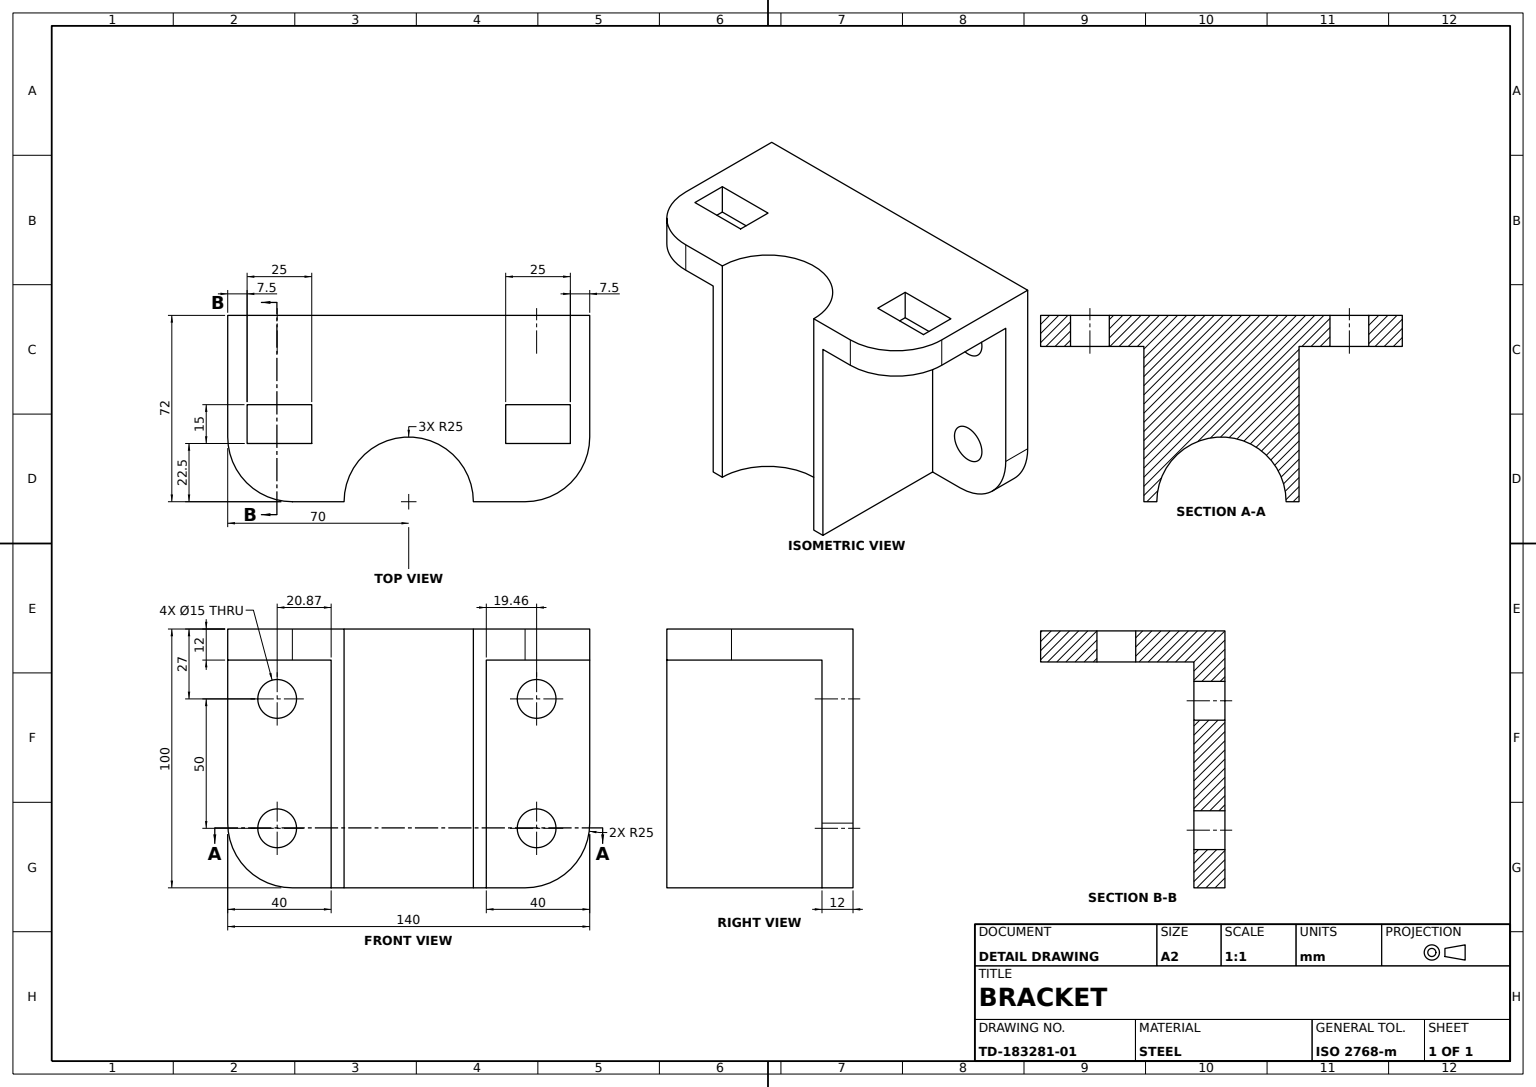
SolidWorks part; units mm, degrees
material "Plain Carbon Steel"
ref_plane "Front Plane" through (0, 0, 0) normal (0, 0, 1) x (1, 0, 0)
ref_plane "Top Plane" through (0, 0, 0) normal (0, 1, 0) x (1, 0, 0)
ref_plane "Right Plane" through (0, 0, 0) normal (1, 0, 0) x (0, 0, -1)
sketch "Base Plate Sketch" plane through (0, 0, 0) normal (0, 0, 1) x (1, 0, 0)
  line L0 (0, 0) -> (0, -75)
  line L2 (140, 0) -> (140, -75)
  line L4 (0, 0) -> (140, 0)
  line L5 (25, -100) -> (115, -100)
  arc A2 (0, -75) -> (25, -100) centre (25, -75) ccw
  arc A3 (115, -100) -> (140, -75) centre (115, -75) ccw
  dimension "D1" = 140
  dimension "D3" = 50
  dimension "D2" = 75
  dimension "D5" = 25
extrude "Base Plate" add sketch "Base Plate Sketch" along normal blind 12
sketch "Side Flange Sketch" plane through (0, 0, 0) normal (0, 1, 0) x (1, 0, 0)
  line L0 (140, -12) -> (140, -47)
  line L4 (0, -12) -> (0, -47)
  line L5 (140, -12) -> (0, -12)
  line L6 (140, 0) -> (0, 0) construction
  line L8 (115, -72) -> (25, -72)
  arc A0 (115, -72) -> (140, -47) centre (115, -47) ccw
  arc A1 (0, -47) -> (25, -72) centre (25, -47) ccw
  dimension "D1" = 25
  dimension "D2" = 72
extrude "Side Flange" add sketch "Side Flange Sketch" against normal blind 12
sketch "Boss Profile Sketch" plane through (0, -12, 0) normal (0, -1, 0) x (1, 0, 0)
  line L0 (25, 72) -> (115, 72) construction
  line L1 (95, 72) -> (100, 72)
  line L2 (100, 72) -> (100, 12)
  line L3 (140, 12) -> (0, 12) construction
  line L4 (45, 72) -> (40, 72)
  line L5 (40, 72) -> (40, 12)
  line L6 (40, 12) -> (100, 12)
  arc A0 (45, 72) -> (95, 72) centre (70, 72) ccw
  dimension "D1" = 25
extrude "Boss 88mm" add sketch "Boss Profile Sketch" along normal blind 88
sketch "Curved Cut Sketch" plane through (0, -12, 0) normal (0, -1, 0) x (1, 0, 0)
  line L0 (45, 72) -> (95, 72)
  arc A0 (45, 72) -> (95, 72) centre (70, 72) ccw
extrude "Curved Cut" cut sketch "Curved Cut Sketch" against normal blind 12
sketch "Slot A Sketch 22.5x7.5" plane through (0, -12, 0) normal (0, -1, 0) x (-1, 0, 0)
  line L0 (-140, -12) -> (-115, -12) construction
  line L1 (-107.5, -49.5) -> (-132.5, -49.5)
  line L2 (-107.5, -49.5) -> (-107.5, -34.5)
  line L3 (-107.5, -34.5) -> (-132.5, -34.5)
  line L4 (-132.5, -49.5) -> (-132.5, -34.5)
  line L5 (-140, -47) -> (-140, -12) construction
  line L6 (-100, -12) -> (-100, -72) construction
  line L7 (-140, -12) -> (-100, -12) construction
  dimension "D1" = 22.5
  dimension "D2" = 7.5
  dimension "D3" = 7.5
  dimension "D4" = 37.5
extrude "Slot A 22.5x7.5" cut sketch "Slot A Sketch 22.5x7.5" against normal blind 12
sketch "Slot B Sketch 7.5x22.5" plane through (0, -12, 0) normal (0, -1, 0) x (-1, 0, 0)
  line L0 (0, -12) -> (0, -47) construction
  line L1 (-7.5, -49.5) -> (-32.5, -49.5)
  line L2 (-7.5, -49.5) -> (-7.5, -34.5)
  line L3 (-7.5, -34.5) -> (-32.5, -34.5)
  line L4 (-32.5, -49.5) -> (-32.5, -34.5)
  line L5 (-40, -12) -> (0, -12) construction
  line L6 (-40, -72) -> (-40, -12) construction
  line L7 (-25, -72) -> (-40, -72) construction
  dimension "D1" = 7.5
  dimension "D2" = 22.5
  dimension "D3" = 7.5
  dimension "D4" = 22.5
extrude "Slot B 7.5x22.5" cut sketch "Slot B Sketch 7.5x22.5" against normal blind 12
sketch "Hole A Sketch Ø15" plane through (0, 0, 12) normal (0, 0, 1) x (1, 0, 0)
  line L0 (140, 0) -> (115, 0) construction
  line L1 (100, -100) -> (100, -12) construction
  circle A0 centre (119.4632, -27) radius 7.5
  circle A1 centre (119.4632, -77) radius 7.5
  dimension "D1" = 15
  dimension "D2" = 15
  dimension "D5" = 15
  dimension "D3" = 50
  dimension "D4" = 27
  dimension "D6" = 19.4632
extrude "Hole A Ø15" cut sketch "Hole A Sketch Ø15" against normal blind 12
sketch "Hole B Sketch Ø15" plane through (0, 0, 12) normal (0, 0, 1) x (1, 0, 0)
  line L0 (25, 0) -> (0, 0) construction
  line L1 (40, -100) -> (40, -12) construction
  circle A0 centre (19.1281, -27) radius 7.5
  circle A1 centre (19.1281, -77) radius 7.5
  dimension "D1" = 15
  dimension "D2" = 15
  dimension "D5" = 15
  dimension "D3" = 27
  dimension "D4" = 50
  dimension "D6" = 20.8719
extrude "Hole B Ø15" cut sketch "Hole B Sketch Ø15" against normal blind 12
